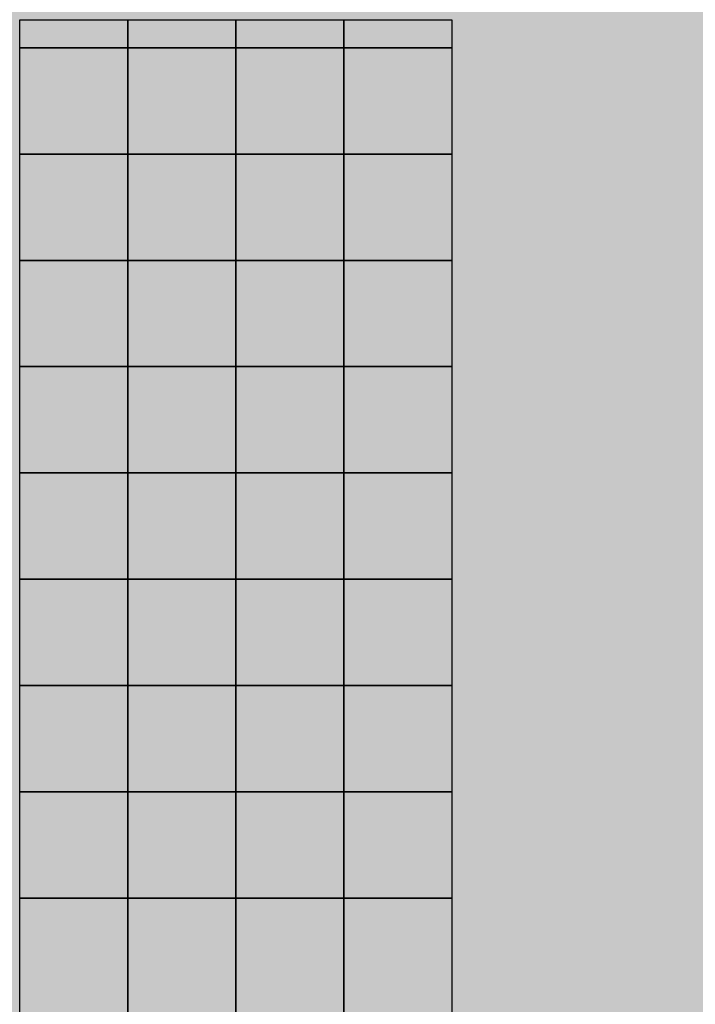
# Model space of a CAD drawing. Units: feet. Extents: x 2695 to 2912, y 795 to 1139.
# Tile 44 of 83: x 2731 to 2769, y 993 to 1048. Entities that reach past the tile are written whole.
import ezdxf

# ---------------------------------------------------------------- set-up
doc = ezdxf.new("R2010")
doc.units = ezdxf.units.FT
for name, color, linetype, lineweight in [('A-ELEV-PATT', 252, 'Continuous', 13), ('A-GLAZ', 4, 'Continuous', 25), ('A-GLAZ-PATT', 254, 'Continuous', 13)]:
    doc.layers.add(name, color=color, linetype=linetype, lineweight=lineweight)

msp = doc.modelspace()

# ---------------------------------------------------------------- hatches: boundary and pattern name
at = {"layer": 'A-ELEV-PATT'}
h = msp.add_hatch(color=256, dxfattribs=at)
h.set_gradient(color1=(147, 149, 152), color2=(147, 149, 152), tint=1)
h.paths.add_polyline_path([(2770.6361, 1118.4096), (2710.6361, 1118.4096), (2710.6361, 1062.9306), (2770.6361, 1062.9306)])
h.paths.add_polyline_path([(2890.6361, 1103.3378), (2770.6361, 1103.3378), (2770.6361, 1062.9306), (2890.6361, 1062.9306)])
h.paths.add_polyline_path([(2730.7081, 1048.1052), (2755.1125, 1048.1052), (2755.1125, 936.9306), (2770.6361, 936.9306), (2770.6361, 1050.3105), (2715.8852, 1050.3105), (2715.8852, 936.9306), (2730.7081, 936.9306)])
h.paths.add_polyline_path([(2890.6361, 1050.3105), (2770.6361, 1050.3105), (2770.6361, 971.9673), (2778.0341, 971.9673), (2778.0341, 1020.8235), (2843.575, 1020.8235), (2843.575, 971.9673), (2890.6361, 971.9673)])
h.paths.add_polyline_path([(2888.1882, 970.7156), (2843.575, 970.7156), (2843.575, 964.8267), (2888.1882, 964.8267)])
h.paths.add_polyline_path([(2888.1882, 964.1328), (2843.575, 964.1328), (2843.575, 956.614), (2888.1882, 956.614)])
h.paths.add_polyline_path([(2888.1882, 955.9202), (2843.575, 955.9202), (2843.575, 949.2892), (2888.1882, 949.2892)])
h.paths.add_polyline_path([(2888.1882, 948.5954), (2843.575, 948.5954), (2843.575, 941.3507), (2888.1882, 941.3507)])
h.paths.add_polyline_path([(2888.1882, 940.6569), (2843.575, 940.6569), (2843.575, 936.9306), (2888.1882, 936.9306)])
h.paths.add_polyline_path([(2890.6361, 970.7156), (2888.9368, 970.7156), (2888.9368, 964.8267), (2890.6361, 964.8267)])
h.paths.add_polyline_path([(2890.6361, 964.1328), (2888.9368, 964.1328), (2888.9368, 956.614), (2890.6361, 956.614)])
h.paths.add_polyline_path([(2890.6361, 955.9202), (2888.9368, 955.9202), (2888.9368, 949.2892), (2890.6361, 949.2892)])
h.paths.add_polyline_path([(2890.6361, 940.6569), (2888.9368, 940.6569), (2888.9368, 936.9306), (2890.6361, 936.9306)])
h.paths.add_polyline_path([(2890.6361, 948.5954), (2888.9368, 948.5954), (2888.9368, 941.3507), (2890.6361, 941.3507)])
h.paths.add_polyline_path([(2772.5216, 970.7156), (2770.6361, 970.7156), (2770.6361, 964.8267), (2772.5216, 964.8267)])
h.paths.add_polyline_path([(2772.5216, 964.1328), (2770.6361, 964.1328), (2770.6361, 956.614), (2772.5216, 956.614)])
h.paths.add_polyline_path([(2772.5216, 955.9202), (2770.6361, 955.9202), (2770.6361, 949.2892), (2772.5216, 949.2892)])
h.paths.add_polyline_path([(2772.5216, 948.5954), (2770.6361, 948.5954), (2770.6361, 941.3507), (2772.5216, 941.3507)])
h.paths.add_polyline_path([(2772.5216, 940.6569), (2770.6361, 940.6569), (2770.6361, 936.9306), (2772.5216, 936.9306)])
h.paths.add_polyline_path([(2778.0341, 940.6569), (2773.2702, 940.6569), (2773.2702, 936.9306), (2778.0341, 936.9306)])
h.paths.add_polyline_path([(2778.0341, 970.7156), (2773.2702, 970.7156), (2773.2702, 964.8267), (2778.0341, 964.8267)])
h.paths.add_polyline_path([(2778.0341, 964.1328), (2773.2702, 964.1328), (2773.2702, 956.614), (2778.0341, 956.614)])
h.paths.add_polyline_path([(2778.0341, 955.9202), (2773.2702, 955.9202), (2773.2702, 949.2892), (2778.0341, 949.2892)])
h.paths.add_polyline_path([(2778.0341, 948.5954), (2773.2702, 948.5954), (2773.2702, 941.3507), (2778.0341, 941.3507)])
h.paths.add_polyline_path([(2810.0407, 940.6569), (2780.0341, 940.6569), (2780.0341, 936.9306), (2810.0407, 936.9306)])
h.paths.add_polyline_path([(2890.6361, 924.3105), (2770.6361, 924.3105), (2770.6361, 810.9306), (2773.5029, 810.9306), (2773.5029, 905.5143), (2805.9398, 905.5143), (2838.3767, 905.5143), (2838.3767, 810.9306), (2890.6361, 810.9306)])
at = {"layer": 'A-GLAZ-PATT'}
h = msp.add_hatch(color=256, dxfattribs=at)
h.set_gradient(color1=(153, 185, 219), color2=(153, 185, 219))
h.paths.add_polyline_path([(2736.8092, 1048.1052), (2730.7081, 1048.1052), (2730.7081, 1046.5179), (2736.8092, 1046.5179)])
h.paths.add_polyline_path([(2742.9103, 1048.1052), (2736.8092, 1048.1052), (2736.8092, 1046.5179), (2742.9103, 1046.5179)])
h.paths.add_polyline_path([(2749.0114, 1048.1052), (2742.9103, 1048.1052), (2742.9103, 1046.5179), (2749.0114, 1046.5179)])
h.paths.add_polyline_path([(2755.1125, 1048.1052), (2749.0114, 1048.1052), (2749.0114, 1046.5179), (2755.1125, 1046.5179)])
h.paths.add_polyline_path([(2755.1125, 1046.5179), (2749.0114, 1046.5179), (2749.0114, 1040.5179), (2755.1125, 1040.5179)])
h.paths.add_polyline_path([(2749.0114, 1046.5179), (2742.9103, 1046.5179), (2742.9103, 1040.5179), (2749.0114, 1040.5179)])
h.paths.add_polyline_path([(2736.8092, 1046.5179), (2730.7081, 1046.5179), (2730.7081, 1040.5179), (2736.8092, 1040.5179)])
h.paths.add_polyline_path([(2742.9103, 1046.5179), (2736.8092, 1046.5179), (2736.8092, 1040.5179), (2742.9103, 1040.5179)])
h.paths.add_polyline_path([(2736.8092, 1040.5179), (2730.7081, 1040.5179), (2730.7081, 1034.5179), (2736.8092, 1034.5179)])
h.paths.add_polyline_path([(2742.9103, 1040.5179), (2736.8092, 1040.5179), (2736.8092, 1034.5179), (2742.9103, 1034.5179)])
h.paths.add_polyline_path([(2749.0114, 1040.5179), (2742.9103, 1040.5179), (2742.9103, 1034.5179), (2749.0114, 1034.5179)])
h.paths.add_polyline_path([(2755.1125, 1040.5179), (2749.0114, 1040.5179), (2749.0114, 1034.5179), (2755.1125, 1034.5179)])
h.paths.add_polyline_path([(2736.8092, 1034.5179), (2730.7081, 1034.5179), (2730.7081, 1028.5179), (2736.8092, 1028.5179)])
h.paths.add_polyline_path([(2749.0114, 1034.5179), (2742.9103, 1034.5179), (2742.9103, 1028.5179), (2749.0114, 1028.5179)])
h.paths.add_polyline_path([(2742.9103, 1034.5179), (2736.8092, 1034.5179), (2736.8092, 1028.5179), (2742.9103, 1028.5179)])
h.paths.add_polyline_path([(2755.1125, 1034.5179), (2749.0114, 1034.5179), (2749.0114, 1028.5179), (2755.1125, 1028.5179)])
h.paths.add_polyline_path([(2755.1125, 1028.5179), (2749.0114, 1028.5179), (2749.0114, 1022.5179), (2755.1125, 1022.5179)])
h.paths.add_polyline_path([(2749.0114, 1028.5179), (2742.9103, 1028.5179), (2742.9103, 1022.5179), (2749.0114, 1022.5179)])
h.paths.add_polyline_path([(2742.9103, 1028.5179), (2736.8092, 1028.5179), (2736.8092, 1022.5179), (2742.9103, 1022.5179)])
h.paths.add_polyline_path([(2736.8092, 1028.5179), (2730.7081, 1028.5179), (2730.7081, 1022.5179), (2736.8092, 1022.5179)])
h.paths.add_polyline_path([(2736.8092, 1022.5179), (2730.7081, 1022.5179), (2730.7081, 1016.5179), (2736.8092, 1016.5179)])
h.paths.add_polyline_path([(2742.9103, 1022.5179), (2736.8092, 1022.5179), (2736.8092, 1016.5179), (2742.9103, 1016.5179)])
h.paths.add_polyline_path([(2749.0114, 1022.5179), (2742.9103, 1022.5179), (2742.9103, 1016.5179), (2749.0114, 1016.5179)])
h.paths.add_polyline_path([(2755.1125, 1022.5179), (2749.0114, 1022.5179), (2749.0114, 1016.5179), (2755.1125, 1016.5179)])
h.paths.add_polyline_path([(2736.8092, 1016.5179), (2730.7081, 1016.5179), (2730.7081, 1010.5179), (2736.8092, 1010.5179)])
h.paths.add_polyline_path([(2742.9103, 1016.5179), (2736.8092, 1016.5179), (2736.8092, 1010.5179), (2742.9103, 1010.5179)])
h.paths.add_polyline_path([(2749.0114, 1016.5179), (2742.9103, 1016.5179), (2742.9103, 1010.5179), (2749.0114, 1010.5179)])
h.paths.add_polyline_path([(2755.1125, 1016.5179), (2749.0114, 1016.5179), (2749.0114, 1010.5179), (2755.1125, 1010.5179)])
h.paths.add_polyline_path([(2755.1125, 1010.5179), (2749.0114, 1010.5179), (2749.0114, 1004.5179), (2755.1125, 1004.5179)])
h.paths.add_polyline_path([(2749.0114, 1010.5179), (2742.9103, 1010.5179), (2742.9103, 1004.5179), (2749.0114, 1004.5179)])
h.paths.add_polyline_path([(2742.9103, 1010.5179), (2736.8092, 1010.5179), (2736.8092, 1004.5179), (2742.9103, 1004.5179)])
h.paths.add_polyline_path([(2736.8092, 1010.5179), (2730.7081, 1010.5179), (2730.7081, 1004.5179), (2736.8092, 1004.5179)])
h.paths.add_polyline_path([(2736.8092, 1004.5179), (2730.7081, 1004.5179), (2730.7081, 998.5179), (2736.8092, 998.5179)])
h.paths.add_polyline_path([(2742.9103, 1004.5179), (2736.8092, 1004.5179), (2736.8092, 998.5179), (2742.9103, 998.5179)])
h.paths.add_polyline_path([(2749.0114, 1004.5179), (2742.9103, 1004.5179), (2742.9103, 998.5179), (2749.0114, 998.5179)])
h.paths.add_polyline_path([(2755.1125, 1004.5179), (2749.0114, 1004.5179), (2749.0114, 998.5179), (2755.1125, 998.5179)])
h.paths.add_polyline_path([(2755.1125, 998.5179), (2749.0114, 998.5179), (2749.0114, 992.5179), (2755.1125, 992.5179)])
h.paths.add_polyline_path([(2749.0114, 998.5179), (2742.9103, 998.5179), (2742.9103, 992.5179), (2749.0114, 992.5179)])
h.paths.add_polyline_path([(2742.9103, 998.5179), (2736.8092, 998.5179), (2736.8092, 992.5179), (2742.9103, 992.5179)])
h.paths.add_polyline_path([(2736.8092, 998.5179), (2730.7081, 998.5179), (2730.7081, 992.5179), (2736.8092, 992.5179)])
h.paths.add_polyline_path([(2736.8092, 992.5179), (2730.7081, 992.5179), (2730.7081, 986.5179), (2736.8092, 986.5179)])
h.paths.add_polyline_path([(2742.9103, 992.5179), (2736.8092, 992.5179), (2736.8092, 986.5179), (2742.9103, 986.5179)])
h.paths.add_polyline_path([(2749.0114, 992.5179), (2742.9103, 992.5179), (2742.9103, 986.5179), (2749.0114, 986.5179)])
h.paths.add_polyline_path([(2755.1125, 992.5179), (2749.0114, 992.5179), (2749.0114, 986.5179), (2755.1125, 986.5179)])
h.paths.add_polyline_path([(2755.1125, 986.5179), (2749.0114, 986.5179), (2749.0114, 980.5179), (2755.1125, 980.5179)])
h.paths.add_polyline_path([(2749.0114, 986.5179), (2742.9103, 986.5179), (2742.9103, 980.5179), (2749.0114, 980.5179)])
h.paths.add_polyline_path([(2742.9103, 986.5179), (2736.8092, 986.5179), (2736.8092, 980.5179), (2742.9103, 980.5179)])
h.paths.add_polyline_path([(2736.8092, 986.5179), (2730.7081, 986.5179), (2730.7081, 980.5179), (2736.8092, 980.5179)])
h.paths.add_polyline_path([(2755.1125, 980.5179), (2749.0114, 980.5179), (2749.0114, 974.5179), (2755.1125, 974.5179)])
h.paths.add_polyline_path([(2749.0114, 980.5179), (2742.9103, 980.5179), (2742.9103, 974.5179), (2749.0114, 974.5179)])
h.paths.add_polyline_path([(2736.8092, 980.5179), (2730.7081, 980.5179), (2730.7081, 974.5179), (2736.8092, 974.5179)])
h.paths.add_polyline_path([(2742.9103, 980.5179), (2736.8092, 980.5179), (2736.8092, 974.5179), (2742.9103, 974.5179)])
h.paths.add_polyline_path([(2736.8092, 974.5179), (2730.7081, 974.5179), (2730.7081, 968.5179), (2736.8092, 968.5179)])
h.paths.add_polyline_path([(2742.9103, 974.5179), (2736.8092, 974.5179), (2736.8092, 968.5179), (2742.9103, 968.5179)])
h.paths.add_polyline_path([(2755.1125, 974.5179), (2749.0114, 974.5179), (2749.0114, 968.5179), (2755.1125, 968.5179)])
h.paths.add_polyline_path([(2749.0114, 974.5179), (2742.9103, 974.5179), (2742.9103, 968.5179), (2749.0114, 968.5179)])
h.paths.add_polyline_path([(2736.8092, 968.5179), (2730.7081, 968.5179), (2730.7081, 962.5179), (2736.8092, 962.5179)])
h.paths.add_polyline_path([(2742.9103, 968.5179), (2736.8092, 968.5179), (2736.8092, 962.5179), (2742.9103, 962.5179)])
h.paths.add_polyline_path([(2749.0114, 968.5179), (2742.9103, 968.5179), (2742.9103, 962.5179), (2749.0114, 962.5179)])
h.paths.add_polyline_path([(2755.1125, 968.5179), (2749.0114, 968.5179), (2749.0114, 962.5179), (2755.1125, 962.5179)])
h.paths.add_polyline_path([(2755.1125, 962.5179), (2749.0114, 962.5179), (2749.0114, 956.5179), (2755.1125, 956.5179)])
h.paths.add_polyline_path([(2749.0114, 962.5179), (2742.9103, 962.5179), (2742.9103, 956.5179), (2749.0114, 956.5179)])
h.paths.add_polyline_path([(2742.9103, 962.5179), (2736.8092, 962.5179), (2736.8092, 956.5179), (2742.9103, 956.5179)])
h.paths.add_polyline_path([(2736.8092, 962.5179), (2730.7081, 962.5179), (2730.7081, 956.5179), (2736.8092, 956.5179)])
h.paths.add_polyline_path([(2736.8092, 956.5179), (2730.7081, 956.5179), (2730.7081, 950.5179), (2736.8092, 950.5179)])
h.paths.add_polyline_path([(2742.9103, 956.5179), (2736.8092, 956.5179), (2736.8092, 950.5179), (2742.9103, 950.5179)])
h.paths.add_polyline_path([(2749.0114, 956.5179), (2742.9103, 956.5179), (2742.9103, 950.5179), (2749.0114, 950.5179)])
h.paths.add_polyline_path([(2755.1125, 956.5179), (2749.0114, 956.5179), (2749.0114, 950.5179), (2755.1125, 950.5179)])
h.paths.add_polyline_path([(2755.1125, 950.5179), (2749.0114, 950.5179), (2749.0114, 944.5179), (2755.1125, 944.5179)])
h.paths.add_polyline_path([(2749.0114, 950.5179), (2742.9103, 950.5179), (2742.9103, 944.5179), (2749.0114, 944.5179)])
h.paths.add_polyline_path([(2742.9103, 950.5179), (2736.8092, 950.5179), (2736.8092, 944.5179), (2742.9103, 944.5179)])
h.paths.add_polyline_path([(2736.8092, 950.5179), (2730.7081, 950.5179), (2730.7081, 944.5179), (2736.8092, 944.5179)])
h.paths.add_polyline_path([(2736.8092, 944.5179), (2730.7081, 944.5179), (2730.7081, 938.5179), (2736.8092, 938.5179)])
h.paths.add_polyline_path([(2742.9103, 944.5179), (2736.8092, 944.5179), (2736.8092, 938.5179), (2742.9103, 938.5179)])
h.paths.add_polyline_path([(2749.0114, 944.5179), (2742.9103, 944.5179), (2742.9103, 938.5179), (2749.0114, 938.5179)])
h.paths.add_polyline_path([(2755.1125, 944.5179), (2749.0114, 944.5179), (2749.0114, 938.5179), (2755.1125, 938.5179)])
h.paths.add_polyline_path([(2755.1125, 938.5179), (2749.0114, 938.5179), (2749.0114, 936.9306), (2755.1125, 936.9306)])
h.paths.add_polyline_path([(2749.0114, 938.5179), (2742.9103, 938.5179), (2742.9103, 936.9306), (2749.0114, 936.9306)])
h.paths.add_polyline_path([(2742.9103, 938.5179), (2736.8092, 938.5179), (2736.8092, 936.9306), (2742.9103, 936.9306)])
h.paths.add_polyline_path([(2736.8092, 938.5179), (2730.7081, 938.5179), (2730.7081, 936.9306), (2736.8092, 936.9306)])

# ---------------------------------------------------------------- linework, layer by layer
at = {"layer": 'A-GLAZ'}
for p, q in [((2736.8092, 936.9306), (2736.8092, 1048.1052)), ((2742.9103, 936.9306), (2742.9103, 1048.1052)), ((2749.0114, 936.9306), (2749.0114, 1048.1052)), ((2749.0114, 1048.1052), (2749.0114, 935.6966)), ((2730.7081, 1046.5179), (2755.1125, 1046.5179)), ((2730.7081, 1040.5179), (2755.1125, 1040.5179)), ((2730.7081, 1034.5179), (2755.1125, 1034.5179)), ((2730.7081, 1028.5179), (2755.1125, 1028.5179)), ((2730.7081, 1022.5179), (2755.1125, 1022.5179)), ((2730.7081, 1016.5179), (2755.1125, 1016.5179)), ((2730.7081, 1010.5179), (2755.1125, 1010.5179)), ((2730.7081, 1004.5179), (2755.1125, 1004.5179)), ((2730.7081, 998.5179), (2755.1125, 998.5179))]:
    msp.add_line(p, q, dxfattribs=at)
msp.add_lwpolyline([(2730.7081, 936.9306), (2730.7081, 1048.1052), (2755.1125, 1048.1052), (2755.1125, 936.9306)], dxfattribs=at)
for points in [[(2730.7081, 1048.1052), (2755.1125, 1048.1052), (2755.1125, 936.9306), (2730.7081, 936.9306)], [(2736.8092, 1048.1052), (2736.8092, 1048.1052), (2736.8092, 936.9306), (2736.8092, 936.9306)], [(2742.9103, 1048.1052), (2742.9103, 1048.1052), (2742.9103, 936.9306), (2742.9103, 936.9306)], [(2749.0114, 1048.1052), (2749.0114, 1048.1052), (2749.0114, 936.9306), (2749.0114, 936.9306)], [(2730.7081, 1046.5179), (2755.1125, 1046.5179), (2755.1125, 1046.5179), (2730.7081, 1046.5179)], [(2730.7081, 1040.5179), (2755.1125, 1040.5179), (2755.1125, 1040.5179), (2730.7081, 1040.5179)], [(2730.7081, 1034.5179), (2755.1125, 1034.5179), (2755.1125, 1034.5179), (2730.7081, 1034.5179)], [(2730.7081, 1028.5179), (2755.1125, 1028.5179), (2755.1125, 1028.5179), (2730.7081, 1028.5179)], [(2730.7081, 1022.5179), (2755.1125, 1022.5179), (2755.1125, 1022.5179), (2730.7081, 1022.5179)], [(2730.7081, 1016.5179), (2755.1125, 1016.5179), (2755.1125, 1016.5179), (2730.7081, 1016.5179)], [(2730.7081, 1010.5179), (2755.1125, 1010.5179), (2755.1125, 1010.5179), (2730.7081, 1010.5179)], [(2730.7081, 1004.5179), (2755.1125, 1004.5179), (2755.1125, 1004.5179), (2730.7081, 1004.5179)], [(2730.7081, 998.5179), (2755.1125, 998.5179), (2755.1125, 998.5179), (2730.7081, 998.5179)]]:
    msp.add_lwpolyline(points, close=True, dxfattribs=at)

doc.saveas('drawing.dxf')
